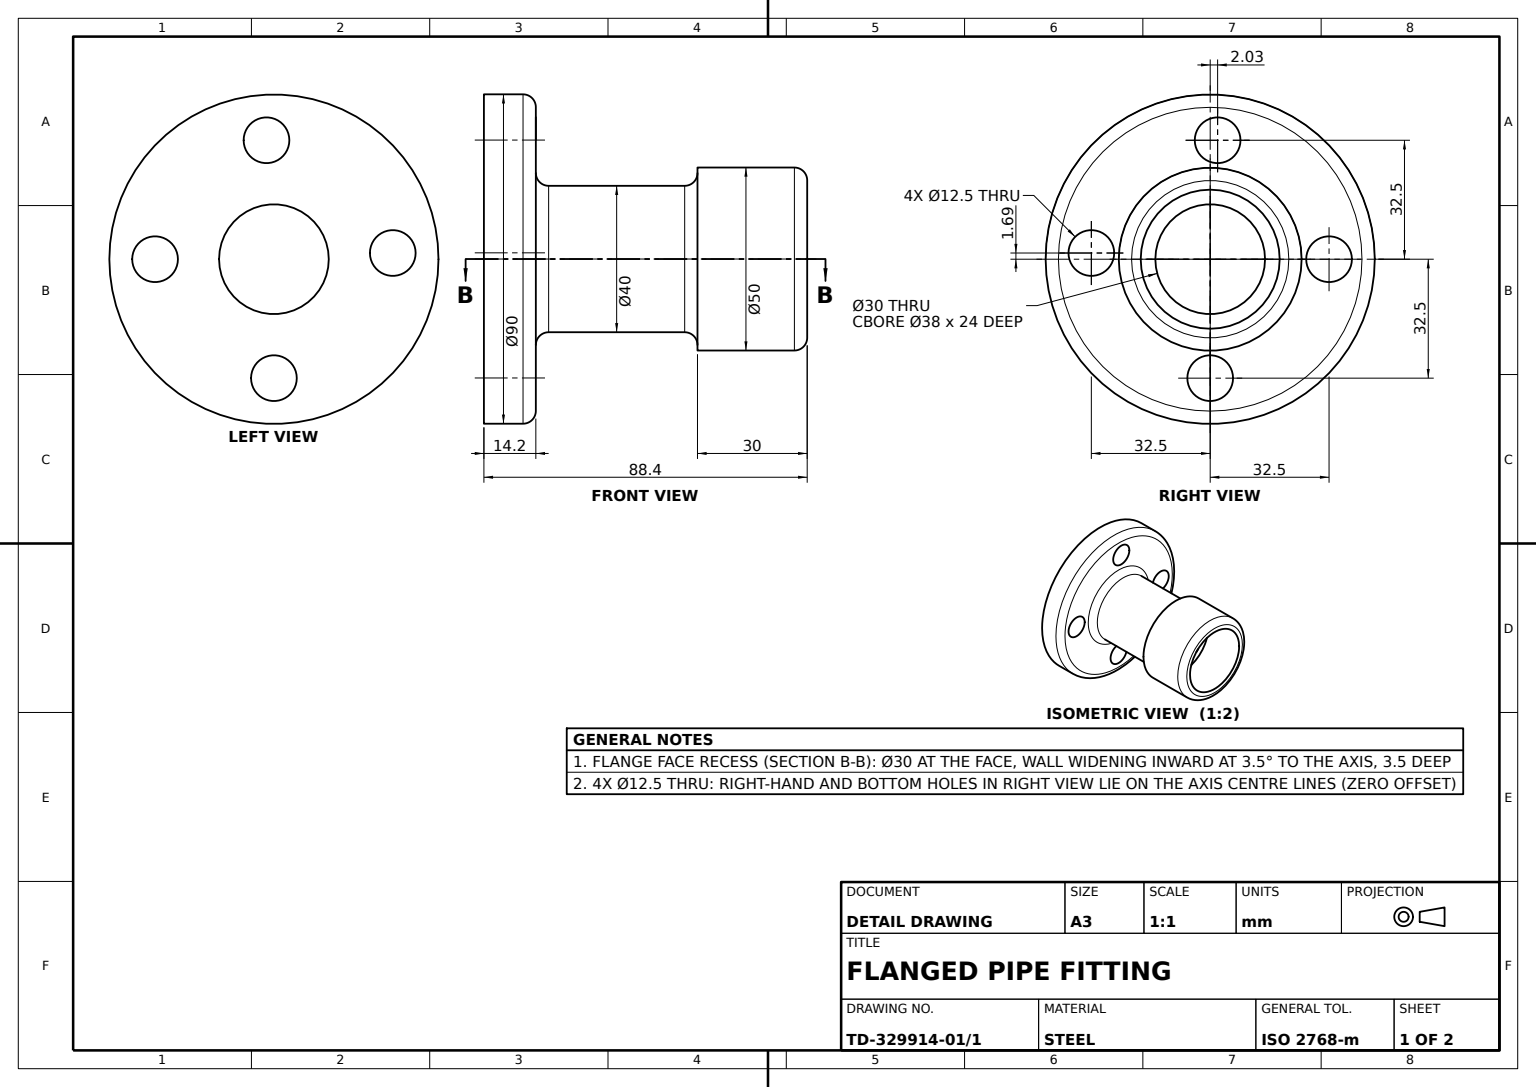
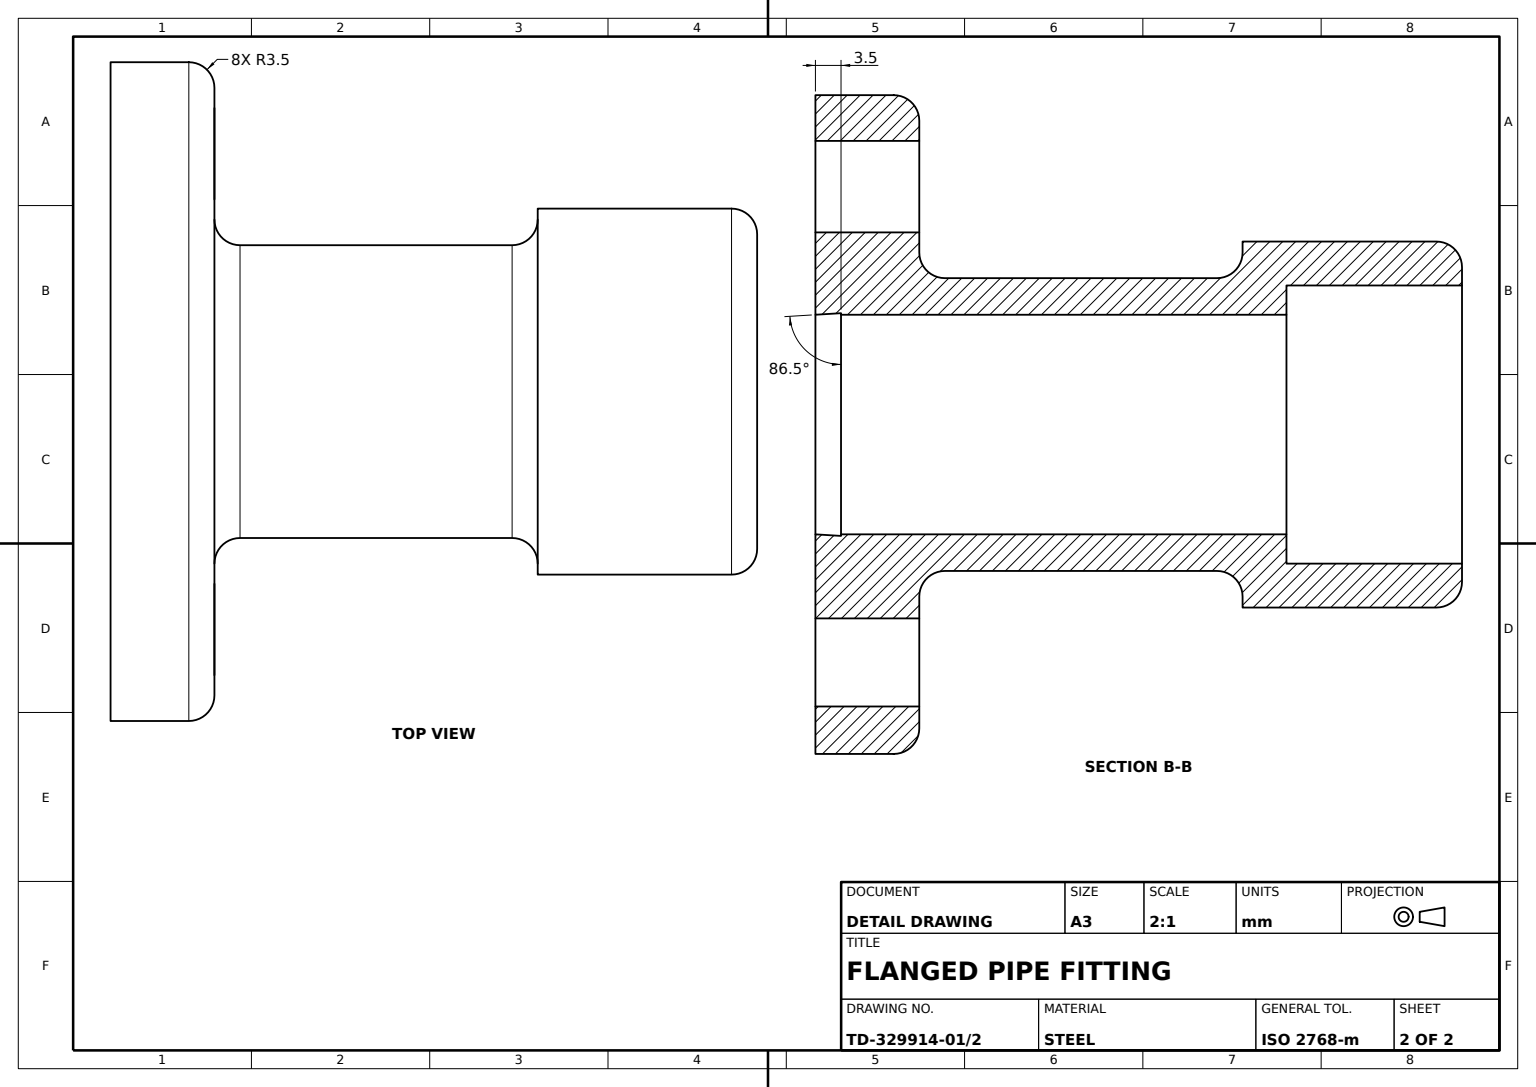
SolidWorks part; units mm, degrees
material "Plain Carbon Steel"
ref_plane "Front Plane" through (0, 0, 0) normal (0, 0, 1) x (1, 0, 0)
ref_plane "Top Plane" through (0, 0, 0) normal (0, 1, 0) x (1, 0, 0)
ref_plane "Right Plane" through (0, 0, 0) normal (1, 0, 0) x (0, 0, -1)
sketch "Flange Sketch" plane through (0, 0, 0) normal (0, 1, 0) x (1, 0, 0)
  circle A0 centre (0, 0) radius 45
  dimension "D1" = 90
extrude "Flange Ø90" add sketch "Flange Sketch" along normal blind 14.2
sketch "Neck Sketch" plane through (0, 14.2, 0) normal (0, 1, 0) x (1, 0, 0)
  circle A0 centre (0, 0) radius 20
  dimension "D1" = 40
extrude "Neck Ø40" add sketch "Neck Sketch" along normal blind 44.2
sketch "Head Sketch" plane through (0, 58.4, 0) normal (0, 1, 0) x (1, 0, 0)
  circle A0 centre (0, 0) radius 25
  dimension "D1" = 50
extrude "Head Ø50" add sketch "Head Sketch" along normal blind 30
sketch "Bolt Hole 1 Sketch" plane through (0, 14.2, 0) normal (0, 1, 0) x (1, 0, 0)
  circle A0 centre (0, 32.5) radius 6.25
  circle A1 centre (0, 0) radius 20 construction
  dimension "D1" = 12.5
  dimension "D2" = 32.5
  dimension "D3" = 32.5
extrude "Bolt Hole 1 Ø12.5" cut sketch "Bolt Hole 1 Sketch" against normal blind 30
sketch "Bolt Hole 2 Sketch" plane through (0, 14.2, 0) normal (0, 1, 0) x (1, 0, 0)
  circle A0 centre (32.5, 0) radius 6.25
  circle A1 centre (0, 0) radius 20 construction
  dimension "D2" = 12.5
  dimension "D1" = 32.5
  dimension "D3" = 32.5
extrude "Bolt Hole 2 Ø12.5" cut sketch "Bolt Hole 2 Sketch" against normal blind 30
sketch "Bolt Hole 3 Sketch" plane through (0, 14.2, 0) normal (0, 1, 0) x (1, 0, 0)
  circle A0 centre (-32.5, 2.0309) radius 6.25
  circle A1 centre (0, 32.5) radius 6.25 construction
  dimension "D1" = 12.5
  dimension "D2" = 32.5
  dimension "D3" = 30.4691
extrude "Bolt Hole 3 Ø12.5" cut sketch "Bolt Hole 3 Sketch" against normal blind 30
sketch "Bolt Hole 4 Sketch" plane through (0, 14.2, 0) normal (0, 1, 0) x (1, 0, 0)
  circle A0 centre (-1.6924, -32.5) radius 6.25
  circle A1 centre (0, 32.5) radius 6.25 construction
  dimension "D1" = 12.5
  dimension "D2" = 32.5
  dimension "D3" = 1.6924
extrude "Bolt Hole 4 Ø12.5" cut sketch "Bolt Hole 4 Sketch" against normal blind 30
sketch "Counterbore Sketch" plane through (0, 88.4, 0) normal (0, 1, 0) x (1, 0, 0)
  circle A0 centre (0, 0) radius 19
  dimension "D1" = 38
extrude "Counterbore Ø38" cut sketch "Counterbore Sketch" against normal blind 12
sketch "Bore Step Sketch" plane through (0, 76.4, 0) normal (0, 1, 0) x (1, 0, 0)
  circle A0 centre (0, 0) radius 19
  dimension "D1" = 38
extrude "Bore Step Depth 12" cut sketch "Bore Step Sketch" against normal blind 12
sketch "Inner Bore Sketch" plane through (0, 64.4, 0) normal (0, 1, 0) x (1, 0, 0)
  circle A0 centre (0, 0) radius 15
  dimension "D1" = 30
extrude "Inner Bore Ø30" cut sketch "Inner Bore Sketch" against normal blind 6
sketch "Neck Bore Sketch" plane through (0, 58.4, 0) normal (0, 1, 0) x (1, 0, 0)
  circle A0 centre (0, 0) radius 15
  dimension "D1" = 30
extrude "Neck Bore" cut sketch "Neck Bore Sketch" against normal blind 44.2
sketch "Bottom Recess Sketch" plane through (0, 0, 0) normal (0, -1, 0) x (1, 0, 0)
  circle A0 centre (0, 0) radius 15
  dimension "D1" = 30
extrude "Bottom Recess Ø30 Drafted" cut sketch "Bottom Recess Sketch" against normal blind 3.5 draft 3.5 draft outward yes
sketch "Through Bore Sketch" plane through (0, 14.2, 0) normal (0, 1, 0) x (1, 0, 0)
  circle A0 centre (0, 0) radius 15
  dimension "D1" = 30
extrude "Through Bore" cut sketch "Through Bore Sketch" against normal blind 80.5
fillet "Flange-Neck Fillet R3.5" radius 3.5 1 edges at (0, 14.2, 20)
fillet "Head Edge Fillet R3.5" radius 3.5 1 edges at (0, 88.4, 25)
fillet "Neck-Head Fillet R3.5" radius 3.5 1 edges at (0, 58.4, 20)
fillet "Flange Edge Fillet R3.5" radius 3.5 1 edges at (0, 14.2, 45)
